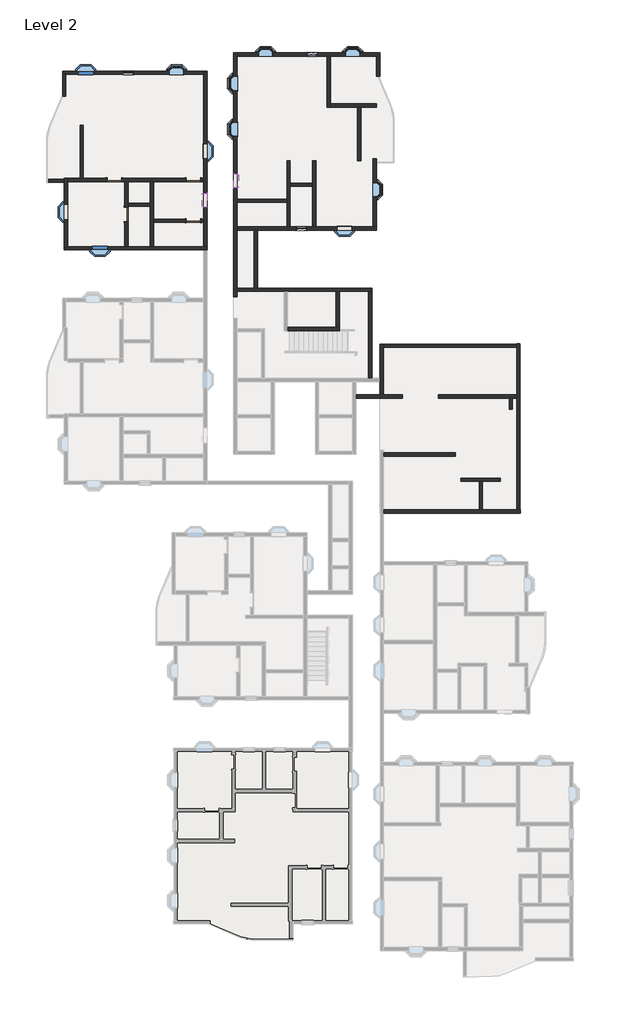
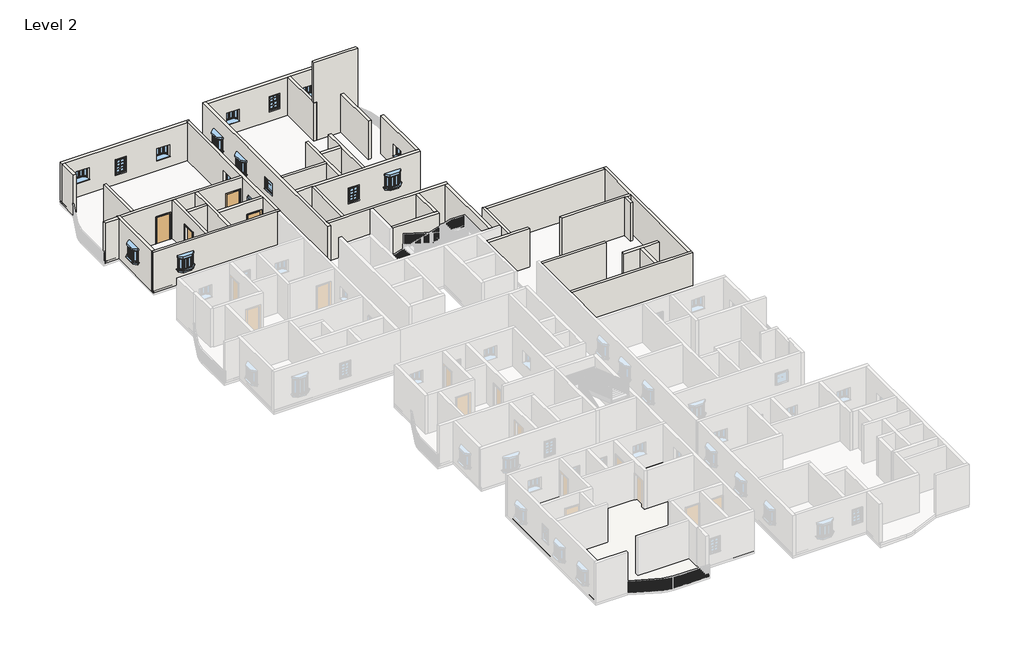
# One storey, part 4 of 14: 40 walls, 16 windows, 4 doors, 1 roof.
# Revit data of these elements (continued)
# Element 28 (IfcWall, "4.5\" p") (continued)
#   Top Offset = 0' - 0"
#   Base Offset = 0' - 0"
#   Unconnected Height = 20' - 0"
#   wall height = 20' - 0"
#   Phase Created = New Construction
#   Base Constraint = Level 2
#   Materials on its faces: "Default Wall", "Brick, Soldier Course"
# Element 30 (IfcWall, "4.5\" p")
#   Top Offset = 0' - 0"
#   Base Offset = 0' - 0"
#   Unconnected Height = 10' - 0"
#   wall height = 10' - 0"
#   Phase Created = New Construction
#   Base Constraint = Level 2
#   Materials on its faces: "Default Wall", "Default Mass Interior Wall"
# Elements 31, 39, 40, 41, 42 (IfcWall, "9\" w")
#   Top Offset = 0' - 0"
#   Base Offset = 0' - 0"
#   wall height = 10' - 0"
#   Phase Created = New Construction
#   Base Constraint = Level 2
#   Top Constraint = Level 3
#   Materials on its faces: "Default Wall"
# Elements 32, 34, 45 (IfcWall, "9\" w")
#   Top Offset = 0' - 0"
#   Base Offset = 0' - 0"
#   wall height = 10' - 0"
#   Phase Created = New Construction
#   Base Constraint = Level 2
#   Top Constraint = Level 3
#   Materials on its faces: "Default Wall", "Brick, Soldier Course"
# Element 33 (IfcWall, "9\" w")
#   Top Offset = 0' - 0"
#   Base Offset = 0' - 0"
#   wall height = 10' - 0"
#   Phase Created = New Construction
#   Base Constraint = Level 2
#   Top Constraint = Level 3
#   Materials on its faces: "Default Wall", "Grass"
# Element 35 (IfcWall, "9\" w")
#   Top Offset = 0' - 0"
#   Base Offset = 0' - 0"
#   wall height = 10' - 0"
#   Phase Created = New Construction
#   Base Constraint = Level 2
#   Top Constraint = Level 3
#   Materials on its faces: "Default Wall", "Parking Stripe"
# Elements 36, 37, 38 (IfcWall, "9\" w")
#   Top Offset = 0' - 0"
#   Base Offset = 0' - 0"
#   wall height = 10' - 0"
#   Phase Created = New Construction
#   Base Constraint = Level 2
#   Top Constraint = Level 3
#   Materials on its faces: "Default Wall", "Window Frame"
# Element 43 (IfcWall, "9\" w")
#   Top Offset = 0' - 0"
#   Base Offset = 0' - 0"
#   wall height = 10' - 0"
#   Phase Created = New Construction
#   Base Constraint = Level 2
#   Top Constraint = Level 3
#   Materials on its faces: "Default Wall", "Wood - Stained", "Default Mass Interior Wall"
# Element 44 (IfcWall, "9\" w")
#   Top Offset = 0' - 0"
#   Base Offset = 0' - 0"
#   wall height = 10' - 0"
#   Phase Created = New Construction
#   Base Constraint = Level 2
#   Top Constraint = Level 3
#   Materials on its faces: "Default Wall", "Parking Stripe", "Brick, Soldier Course"
# Element 46 (IfcWindow, "910x910mm")
#   Mark = "61"
#   Phase Created = New Construction
#   Materials on its faces: "Window Frame", "Glass"
# Element 47 (IfcWindow, "910x910mm")
#   Mark = "62"
#   Phase Created = New Construction
#   Materials on its faces: "Window Frame", "Glass"
# Element 48 (IfcWindow, "910x910mm")
#   Mark = "63"
#   Phase Created = New Construction
#   Materials on its faces: "Window Frame", "Glass"
# Element 49 (IfcWindow, "910x910mm")
#   Mark = "93"
#   Phase Created = New Construction
#   Materials on its faces: "Window Frame", "Glass"
# Element 50 (IfcWindow, "910x910mm")
#   Mark = "94"
#   Phase Created = New Construction
#   Materials on its faces: "Window Frame", "Glass"
# Element 51 (IfcWindow, "910x910mm")
#   Mark = "277"
#   Phase Created = New Construction
#   Materials on its faces: "Window Frame", "Glass"
# Element 52 (IfcWindow, "910x910mm")
#   Mark = "278"
#   Phase Created = New Construction
#   Materials on its faces: "Window Frame", "Glass"
# Element 53 (IfcWindow, "910x910mm")
#   Mark = "289"
#   Phase Created = New Construction
#   Materials on its faces: "Window Frame", "Glass"
# Element 54 (IfcWindow, "910x910mm")
#   Mark = "290"
#   Phase Created = New Construction
#   Materials on its faces: "Window Frame", "Glass"
# Element 55 (IfcWindow, "910x910mm")
#   Mark = "95"
#   Phase Created = New Construction
#   Materials on its faces: "Window Frame", "Glass"
# Element 56 (IfcWindow, "910x910mm")
#   Mark = "96"
#   Phase Created = New Construction
#   Materials on its faces: "Window Frame", "Glass"
# Element 57 (IfcWindow, "Window-Double-Hung : 26\" x 42\"")
#   Mark = "279"
#   Window Inset = 0' - 0"
#   Interior Wall Closure = 0' - 1 1/2"
#   Frame Extension = 0' - 1 1/4"
#   Exterior Wall Closure = 0' - 0 1/2"
#   Interior Trim Visibility = yes
#   Indicator Visibility = yes
#   Exterior Trim Visibility = yes
#   Phase Created = New Construction
#   Materials on its faces: "Wood - Stained", "Glass", "Clad - White"
# Element 58 (IfcWindow, "Window-Double-Hung : 26\" x 42\"")
#   Mark = "291"
#   Window Inset = 0' - 0"
#   Interior Wall Closure = 0' - 1 1/2"
#   Frame Extension = 0' - 1 1/4"
#   Exterior Wall Closure = 0' - 0 1/2"
#   Interior Trim Visibility = yes
#   Indicator Visibility = yes
#   Exterior Trim Visibility = yes
#   Phase Created = New Construction
#   Materials on its faces: "Wood - Stained", "Glass", "Clad - White"
# Element 59 (IfcWindow, "Window-Double-Hung : 26\" x 42\"")
#   Mark = "114"
#   Window Inset = 0' - 0"
#   Interior Wall Closure = 0' - 1 1/2"
#   Frame Extension = 0' - 1 1/4"
#   Exterior Wall Closure = 0' - 0 1/2"
#   Interior Trim Visibility = yes
#   Indicator Visibility = yes
#   Exterior Trim Visibility = yes
#   Phase Created = New Construction
#   Materials on its faces: "Wood - Stained", "Glass", "Clad - White"
# Element 60 (IfcWindow, "Windows_Sgl_w-Glazing_Bars : 910x910mm")
#   Mark = "97"
#   Phase Created = New Construction
#   Materials on its faces: "Window Frame", "Glass"
# Element 61 (IfcWindow, "Windows_Sgl_w-Glazing_Bars : 910x910mm")
#   Mark = "101"
#   Phase Created = New Construction
#   Materials on its faces: "Window Frame", "Glass"
# Materials
#   "Door - Panel": class "Wood", colour RGB 210 159 95, transparency 0, Cost = 0
#   "Door - Frame": colour RGB 118 70 51, transparency 0, Cost = 0
#   "Window Frame": colour RGB 249 249 249, transparency 0
#   "Glass": class "Glass", colour RGB 0 128 192, transparency 0.75, Description = "Soda Lime Glass", Cost = 0
#   "Wood - Stained": class "Wood", colour RGB 224 178 126, transparency 0, Cost = 0
#   "Clad - White": class "Wood", colour RGB 242 242 238, transparency 0, Cost = 0
#   "Default Roof": colour RGB 88 101 114, transparency 0, Cost = 0
#   "Default Wall": colour RGB 128 128 128, transparency 0, Cost = 0
#   "Earth": class "Generic", colour RGB 97 75 62, transparency 0, Description = "Soil", Cost = 0
#   "Parking Stripe": class "Paint", colour RGB 250 250 91, transparency 0, Cost = 0
#   "Carpet (1)": class "Carpet", colour RGB 124 80 67, transparency 0, Description = "Interior finish", Cost = 0
#   "Brick, Soldier Course": class "Masonry", colour RGB 170 98 104, transparency 0, Description = "Common brick soldier coursed", Cost = 0
#   "Default Mass Interior Wall": class "Generic", colour RGB 195 229 126, transparency 0, Cost = 0
#   "Grass": class "Generic", colour RGB 104 137 66, transparency 0, Description = "Physical material.", Cost = 0
